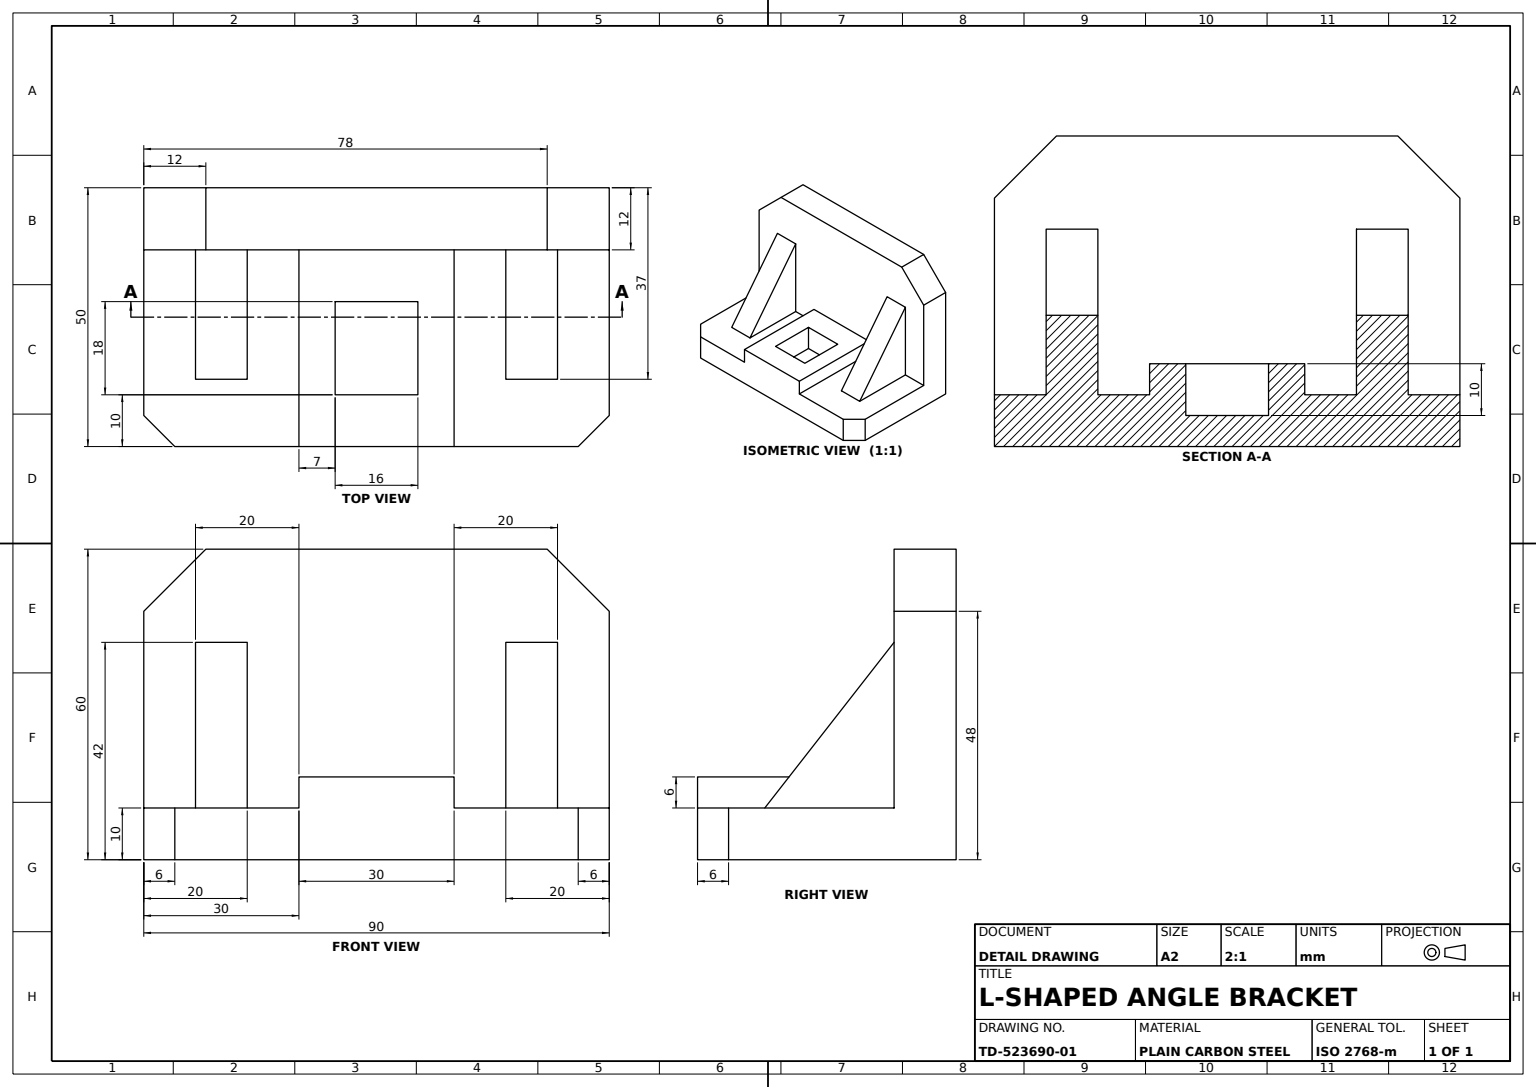
SolidWorks part; units mm, degrees
material "Plain Carbon Steel"
ref_plane "Front Plane" through (0, 0, 0) normal (0, 0, 1) x (1, 0, 0)
ref_plane "Top Plane" through (0, 0, 0) normal (0, 1, 0) x (1, 0, 0)
ref_plane "Right Plane" through (0, 0, 0) normal (1, 0, 0) x (0, 0, -1)
sketch "Back Wall Profile" plane through (0, 0, 0) normal (0, 0, 1) x (1, 0, 0)
  line L0 (0, 0) -> (0, 48)
  line L1 (12, 60) -> (78, 60)
  line L2 (90, 48) -> (90, 0)
  line L3 (90, 0) -> (0, 0)
  line L10 (0, 48) -> (12, 60)
  line L11 (90, 48) -> (78, 60)
  dimension "D1" = 12
  dimension "D2" = 78
  dimension "D3" = 48
  dimension "D4" = 60
extrude "Back Wall" add sketch "Back Wall Profile" along normal blind 12
sketch "Base Plate Profile" plane through (0, 0, 0) normal (0, -1, 0) x (1, 0, 0)
  line L3 (90, 12) -> (0, 12)
  line L8 (0, 12) -> (0, 44)
  line L9 (90, 12) -> (90, 44)
  line L10 (6, 50) -> (84, 50)
  line L13 (90, 12) -> (90, 0) construction
  line L16 (0, 44) -> (6, 50)
  line L17 (90, 44) -> (84, 50)
  line L18 (0, 0) -> (90, 0) construction
  dimension "D1" = 6
  dimension "D2" = 44
extrude "Base Plate" add sketch "Base Plate Profile" against normal blind 10
sketch "Square Pad Profile 30x30" plane through (0, 10, 0) normal (0, 1, 0) x (1, 0, 0)
  line L0 (0, -12) -> (90, -12) construction
  line L1 (30, -12) -> (60, -12)
  line L2 (30, -12) -> (30, -50)
  line L3 (30, -50) -> (60, -50)
  line L4 (60, -12) -> (60, -50)
  line L5 (84, -50) -> (6, -50) construction
  line L6 (0, -44) -> (0, -12) construction
  dimension "D1" = 30
  dimension "D2" = 30
extrude "Square Pad 30x30" add sketch "Square Pad Profile 30x30" along normal blind 6
sketch "Pad Pocket Profile" plane through (0, 16, 0) normal (0, 1, 0) x (1, 0, 0)
  line L0 (60, -50) -> (60, -12) construction
  line L1 (37, -22) -> (53, -22)
  line L2 (37, -22) -> (37, -40)
  line L3 (37, -40) -> (53, -40)
  line L4 (53, -22) -> (53, -40)
  line L5 (60, -12) -> (30, -12) construction
  line L6 (30, -50) -> (60, -50) construction
  point P8 (45, -12)
  dimension "D1" = 16
  dimension "D2" = 7
  dimension "D3" = 10
  dimension "D4" = 10
extrude "Pad Pocket" cut sketch "Pad Pocket Profile" against normal blind 10
sketch "Rib 1 Profile" plane through (0, 0, 0) normal (-1, 0, 0) x (0, 0, 1)
  line L0 (12, 10) -> (12, 42)
  line L1 (12, 48) -> (12, 10) construction
  line L2 (12, 10) -> (37, 10)
  line L3 (12, 10) -> (50, 10) construction
  line L4 (37, 10) -> (12, 42)
  line L5 (0, 48) -> (0, 0) construction
  line L6 (44, 0) -> (0, 0) construction
  dimension "D1" = 37
  dimension "D2" = 42
extrude "Rib 1" add sketch "Rib 1 Profile" against normal blind 20
sketch "Rib 2 Profile" plane through (90, 0, 0) normal (1, 0, 0) x (0, 0, -1)
  line L0 (-12, 10) -> (-12, 42)
  line L1 (-12, 10) -> (-37, 10)
  line L4 (-50, 10) -> (-12, 10) construction
  line L5 (-37, 10) -> (-12, 42) construction
  line L6 (-37, 10) -> (-12, 42)
extrude "Rib 2" add sketch "Rib 2 Profile" against normal blind 20
sketch "Triangular Cut 2 Profile" plane through (90, 0, 0) normal (1, 0, 0) x (0, 0, -1)
  line L0 (-12, 42) -> (-12, 10)
  line L1 (-12, 10) -> (-37, 10)
  line L2 (-44, 0) -> (0, 0) construction
  line L4 (-37, 10) -> (-12, 42)
  dimension "D1" = 37
  dimension "D2" = 10
extrude "Triangular Cut 2" cut sketch "Triangular Cut 2 Profile" against normal blind 10
sketch "Triangular Cut 1 Profile" plane through (0, 0, 0) normal (-1, 0, 0) x (0, 0, 1)
  line L0 (12, 42) -> (12, 10)
  line L1 (12, 10) -> (37, 10)
  line L4 (37, 10) -> (12, 42)
  dimension "D1" = 25
  dimension "D2" = 32
extrude "Triangular Cut 1" cut sketch "Triangular Cut 1 Profile" against normal blind 10
